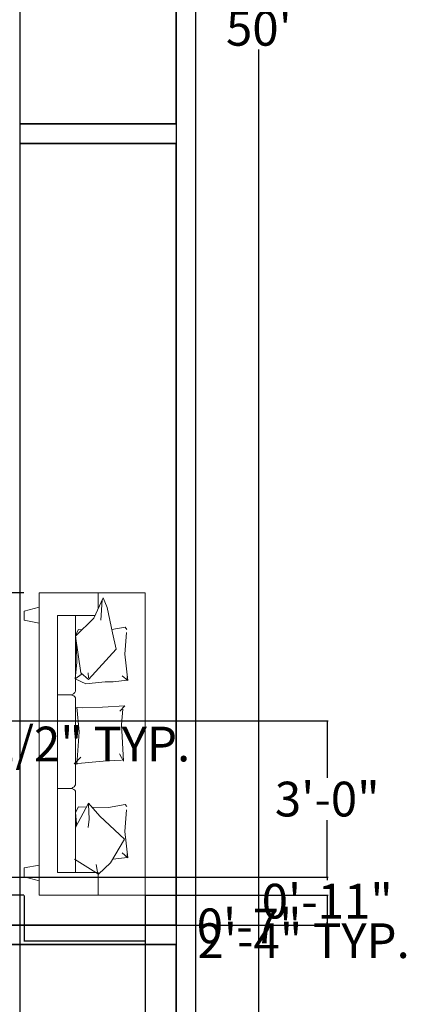
# Model space of a CAD drawing. Units: inches. Extents: x -26 to 385, y 12 to 697.
# Tile 11 of 13: x 285 to 374, y 130 to 356. Entities that reach past the tile are written whole.
import ezdxf

# ---------------------------------------------------------------- set-up
doc = ezdxf.new("R2010")
doc.units = ezdxf.units.IN
doc.header["$MEASUREMENT"] = 0
for name, color, linetype, lineweight in [('A-ANNO-DIMS', 4, 'Continuous', 18), ('A-FLOR-STRS', 215, 'Continuous', 18), ('A-WALL', 40, 'Continuous', 35), ('C-PROP', 40, 'Continuous', 25), ('Furniture', 210, 'Continuous', 15)]:
    doc.layers.add(name, color=color, linetype=linetype, lineweight=lineweight)
doc.styles.get("Standard").update_dxf_attribs({"font": 'italic8.shx'})
doc.dimstyles.get("Standard").update_dxf_attribs({"dimtxt": 8, "dimasz": 0.18, "dimexe": 0.18, "dimexo": 0.0625, "dimgap": 0.09, "dimtad": 0, "dimtih": 1, "dimtoh": 1, "dimdec": 4, "dimzin": 0, "dimdsep": 46, "dimlunit": 3, "dimtxsty": 'Standard', "dimcen": 0.09, "dimclrd": 2, "dimclre": 3, "dimclrt": 6, "dimadec": 0, "dimazin": 0, "dimtfac": 1, "dimtdec": 4, "dimtofl": 0, "dimtmove": 0, "dimatfit": 3, "dimfxl": 1, "dimtolj": 1, "dimtzin": 0, "dimarcsym": 0})

# ---------------------------------------------------------------- blocks, each defined once
blk = doc.blocks.new('*D2')
at = {"layer": 'A-ANNO-DIMS', "color": 0, "lineweight": -2, "transparency": 16777216}
for p, q in [((325.19, 654.38), (339.84, 654.38)), ((339.66, 654.2), (339.66, 359.23)), ((339.66, 54.56), (339.66, 349.53)), ((325.19, 54.38), (339.84, 54.38))]:
    blk.add_line(p, q, dxfattribs=at)
at = {"layer": 'A-ANNO-DIMS', "color": 0, "transparency": 16777216}
for points in [[(339.63, 654.2), (339.69, 654.2), (339.66, 654.38)], [(339.63, 54.56), (339.69, 54.56), (339.66, 54.38)]]:
    blk.add_solid(points, dxfattribs=at)
at = {"layer": 'Defpoints', "color": 0, "transparency": 16777216}
for p in [(325.13, 654.38), (325.13, 54.38), (339.66, 54.38)]:
    blk.add_point(p, dxfattribs=at)
at = {"layer": 'A-ANNO-DIMS', "color": 0, "transparency": 16777216, "insert": (339.66, 354.38), "char_height": 8, "attachment_point": 5}
blk.add_mtext("\\A1;50'", dxfattribs=at)
blk = doc.blocks.new('SOFA-THREE-SEAT')
for p, q in [((-5.22, 20.2), (64.44, 20.2)), ((-5.22, 20.2), (-5.22, -4.18)), ((64.44, 20.2), (64.44, -4.18)), ((2.7, 15.63), (3.2, 15.97)), ((3.92, 15.91), (8.89, 15.54)), ((8.89, 15.54), (14.99, 16.19)), ((14.99, 16.19), (13.87, 14.88)), ((14.06, 16.09), (14.9, 16.1)), ((14.9, 16.1), (15.27, 12.82)), ((43.52, 15.63), (44.02, 15.97)), ((44.74, 15.91), (49.71, 15.54)), ((49.71, 15.54), (55.81, 16.19)), ((55.81, 16.19), (54.69, 14.88)), ((54.88, 16.09), (55.72, 16.1)), ((55.72, 16.1), (56.09, 12.82)), ((3.23, 12.52), (2.7, 15.63)), ((21.11, 10.37), (20.83, 15.51)), ((20.83, 15.51), (22.04, 14.39)), ((21.58, 15.04), (25.13, 14.76)), ((25.13, 14.76), (33.53, 15.23)), ((33.53, 15.23), (31.85, 14.29)), ((33.35, 14.76), (33.44, 11.4)), ((44.18, 11.79), (43.52, 15.63)), ((46.2, 9.78), (51.51, 15.49)), ((51.51, 15.49), (56.95, 12.22)), ((-1.8, 11.46), (-4.04, 10.53)), ((3.97, 12.67), (-1.8, 11.46)), ((7.78, 13.51), (3.97, 12.67)), ((14.76, 7.19), (7.78, 13.51)), ((15.27, 12.82), (15.27, 11.04)), ((33.44, 11.4), (34.19, 3.84)), ((44.12, 7.99), (44.18, 11.79)), ((56.09, 12.82), (56.09, 12.74)), ((56.95, 12.22), (59.54, 9.5)), ((-5.22, 9.4), (-1.58, 9.4)), ((-4.04, 10.53), (0.62, 8.39)), ((-3.57, 10.35), (1.08, 9.97)), ((15.27, 11.04), (15.74, 6.54)), ((21.3, 5.71), (21.11, 10.37)), ((43.2, 7.19), (46.2, 9.78)), ((59.54, 9.5), (56.14, 3.93)), ((59.13, 9.23), (57.36, 8.96)), ((59.21, 9.4), (59.21, 0)), ((59.21, 9.4), (64.44, 9.4)), ((0, 8.68), (0, 0)), ((0.62, 8.39), (4.8, 4.21)), ((14.39, 7.19), (13.18, 7.09)), ((13.18, 5.42), (14.76, 7.19)), ((48.79, 4.2), (43.2, 7.19)), ((43.48, 7.19), (46.88, 7.33)), ((46.88, 7.33), (48.79, 7.06)), ((3.26, 4.85), (3.27, 5.74)), ((4.57, 4.19), (3.26, 4.85)), ((4.8, 4.21), (13.18, 5.42)), ((14.62, 4.1), (13.47, 5.75)), ((15.74, 6.54), (14.62, 4.1)), ((21.11, 4.5), (26.81, 5.06)), ((21.2, 4.4), (21.3, 5.71)), ((26.81, 5.06), (34.28, 4.5)), ((34.19, 3.84), (32.6, 5.43)), ((44.08, 4.85), (44.11, 6.71)), ((45.4, 4.19), (44.08, 4.85)), ((0, 4.18), (17.44, 4.18)), ((7.11, 4.38), (4.57, 4.19)), ((10.86, 4.47), (7.11, 4.38)), ((14.62, 4.1), (10.86, 4.47)), ((18.3, 3.23), (18.3, 0)), ((18.93, 4.18), (38.96, 4.18)), ((39.82, 3.23), (39.82, 0)), ((40.44, 4.18), (59.21, 4.18)), ((47.93, 4.38), (45.4, 4.19)), ((48.43, 4.39), (47.93, 4.38)), ((0, 0), (59.21, 0)), ((-5.22, -4.18), (64.44, -4.18)), ((-1.91, -4.18), (-1.01, -7.66)), ((1.75, -4.18), (1.07, -7.66)), ((57.47, -4.18), (58.14, -7.66)), ((61.12, -4.18), (60.22, -7.66)), ((-1.01, -7.66), (1.07, -7.66)), ((58.14, -7.66), (60.22, -7.66))]:
    blk.add_line(p, q)
for points, knots in [([(17.44, 4.18), (17.62, 4.1), (18, 3.87), (18.2, 3.46), (18.3, 3.23)], [15.247039, 15.247039, 15.247039, 15.247039, 32.166322, 53.547435, 53.547435, 53.547435, 53.547435]), ([(18.3, 3.22), (18.36, 3.42), (18.48, 3.8), (18.78, 4.06), (18.93, 4.18)], [5.353258, 5.353258, 5.353258, 5.353258, 23.098733, 39.167876, 39.167876, 39.167876, 39.167876]), ([(38.96, 4.18), (39.14, 4.1), (39.51, 3.87), (39.71, 3.46), (39.82, 3.23)], [15.247039, 15.247039, 15.247039, 15.247039, 32.166322, 53.547435, 53.547435, 53.547435, 53.547435]), ([(39.82, 3.22), (39.87, 3.42), (39.99, 3.8), (40.29, 4.06), (40.44, 4.18)], [5.353258, 5.353258, 5.353258, 5.353258, 23.098733, 39.167876, 39.167876, 39.167876, 39.167876])]:
    blk.add_open_spline(points, degree=3, knots=knots)
blk = doc.blocks.new('*D11')
at = {"layer": 'A-ANNO-DIMS', "color": 3, "lineweight": -2, "transparency": 16777216}
for p, q in [((285.56, 224.4), (274.99, 224.4)), ((285.56, 154.74), (274.99, 154.74))]:
    blk.add_line(p, q, dxfattribs=at)
at = {"layer": 'A-ANNO-DIMS', "color": 2, "lineweight": -2, "transparency": 16777216}
for p, q in [((275.17, 224.22), (275.17, 195.75)), ((275.17, 154.92), (275.17, 183.38))]:
    blk.add_line(p, q, dxfattribs=at)
at = {"layer": 'A-ANNO-DIMS', "color": 2, "transparency": 16777216}
for points in [[(275.14, 224.22), (275.2, 224.22), (275.17, 224.4)], [(275.14, 154.92), (275.2, 154.92), (275.17, 154.74)]]:
    blk.add_solid(points, dxfattribs=at)
at = {"layer": 'Defpoints', "color": 0, "transparency": 16777216}
for p in [(285.62, 224.4), (275.17, 154.74), (285.62, 154.74)]:
    blk.add_point(p, dxfattribs=at)
at = {"layer": 'A-ANNO-DIMS', "color": 6, "transparency": 16777216, "insert": (275.17, 189.57), "char_height": 8, "attachment_point": 5}
blk.add_mtext('\\A1;SOFA 5\'-9 1/2" TYP.', dxfattribs=at)
blk = doc.blocks.new('*D12')
at = {"layer": 'A-ANNO-DIMS', "color": 3, "lineweight": -2, "transparency": 16777216}
for p, q in [((285.62, 154.68), (285.62, 144.11)), ((313.49, 154.68), (313.49, 144.11))]:
    blk.add_line(p, q, dxfattribs=at)
at = {"layer": 'A-ANNO-DIMS', "color": 2, "lineweight": -2, "transparency": 16777216}
for p, q in [((285.8, 144.29), (313.31, 144.29)), ((313.49, 144.29), (313.67, 144.29))]:
    blk.add_line(p, q, dxfattribs=at)
at = {"layer": 'A-ANNO-DIMS', "color": 2, "transparency": 16777216}
for points in [[(285.8, 144.32), (285.8, 144.26), (285.62, 144.29)], [(313.31, 144.32), (313.31, 144.26), (313.49, 144.29)]]:
    blk.add_solid(points, dxfattribs=at)
at = {"layer": 'Defpoints', "color": 0, "transparency": 16777216}
for p in [(285.62, 154.74), (313.49, 154.74), (313.49, 144.29)]:
    blk.add_point(p, dxfattribs=at)
at = {"layer": 'A-ANNO-DIMS', "color": 6, "transparency": 16777216, "insert": (349.95, 144.29), "char_height": 8, "attachment_point": 5}
blk.add_mtext('\\A1;2\'-4" TYP.', dxfattribs=at)
blk = doc.blocks.new('*D25')
at = {"layer": 'A-ANNO-DIMS', "color": 3, "lineweight": -2, "transparency": 16777216}
for p, q in [((284.629322, 368.316588), (284.629322, 23.949088)), ((320.629322, 368.316588), (320.629322, 23.949088))]:
    blk.add_line(p, q, dxfattribs=at)
at = {"layer": 'A-ANNO-DIMS', "color": 2, "lineweight": -2, "transparency": 16777216}
for p, q in [((284.449322, 24.129088), (284.269322, 24.129088)), ((320.809322, 24.129088), (320.989322, 24.129088))]:
    blk.add_line(p, q, dxfattribs=at)
at = {"layer": 'A-ANNO-DIMS', "color": 2, "transparency": 16777216}
for points in [[(284.449322, 24.159088), (284.449322, 24.099088), (284.629322, 24.129088)], [(320.809322, 24.159088), (320.809322, 24.099088), (320.629322, 24.129088)]]:
    blk.add_solid(points, dxfattribs=at)
at = {"layer": 'Defpoints', "color": 0, "transparency": 16777216}
for p in [(284.629322, 368.379088), (320.629322, 368.379088), (320.629322, 24.129088)]:
    blk.add_point(p, dxfattribs=at)
at = {"layer": 'A-ANNO-DIMS', "color": 6, "transparency": 16777216, "insert": (302.629322, 24.129088), "char_height": 8, "attachment_point": 5}
blk.add_mtext('\\A1;3\'-0"', dxfattribs=at)
blk = doc.blocks.new('*D28')
at = {"layer": 'A-ANNO-DIMS', "color": 3, "lineweight": -2, "transparency": 16777216}
for p, q in [((141.69, 194.9), (355.56, 194.9)), ((141.69, 158.9), (355.56, 158.9))]:
    blk.add_line(p, q, dxfattribs=at)
at = {"layer": 'A-ANNO-DIMS', "color": 2, "lineweight": -2, "transparency": 16777216}
for p, q in [((355.38, 194.72), (355.38, 181.76)), ((355.38, 159.08), (355.38, 172.05))]:
    blk.add_line(p, q, dxfattribs=at)
at = {"layer": 'A-ANNO-DIMS', "color": 2, "transparency": 16777216}
for points in [[(355.35, 194.72), (355.41, 194.72), (355.38, 194.9)], [(355.35, 159.08), (355.41, 159.08), (355.38, 158.9)]]:
    blk.add_solid(points, dxfattribs=at)
at = {"layer": 'Defpoints', "color": 0, "transparency": 16777216}
for p in [(141.63, 194.9), (355.38, 194.9), (141.63, 158.9)]:
    blk.add_point(p, dxfattribs=at)
at = {"layer": 'A-ANNO-DIMS', "color": 6, "transparency": 16777216, "insert": (355.38, 176.9), "char_height": 8, "attachment_point": 5}
blk.add_mtext('\\A1;3\'-0"', dxfattribs=at)
blk = doc.blocks.new('*D31')
at = {"layer": 'A-ANNO-DIMS', "color": 3, "lineweight": -2, "transparency": 16777216}
for p, q in [((239.89, 166.08), (239.89, 23.95)), ((263.51, 166.08), (263.51, 23.95))]:
    blk.add_line(p, q, dxfattribs=at)
at = {"layer": 'A-ANNO-DIMS', "color": 2, "lineweight": -2, "transparency": 16777216}
for p, q in [((240.07, 24.13), (263.33, 24.13)), ((263.51, 24.13), (263.69, 24.13))]:
    blk.add_line(p, q, dxfattribs=at)
at = {"layer": 'A-ANNO-DIMS', "color": 2, "transparency": 16777216}
for points in [[(240.07, 24.16), (240.07, 24.1), (239.89, 24.13)], [(263.33, 24.16), (263.33, 24.1), (263.51, 24.13)]]:
    blk.add_solid(points, dxfattribs=at)
at = {"layer": 'Defpoints', "color": 0, "transparency": 16777216}
for p in [(239.89, 166.14), (263.51, 166.14), (263.51, 24.13)]:
    blk.add_point(p, dxfattribs=at)
at = {"layer": 'A-ANNO-DIMS', "color": 6, "transparency": 16777216, "insert": (296.73, 24.13), "char_height": 8, "attachment_point": 5}
blk.add_mtext('\\A1;1\'-11 1/2"', dxfattribs=at)
blk = doc.blocks.new('*D35')
at = {"layer": 'A-ANNO-DIMS', "color": 3, "lineweight": -2, "transparency": 16777216}
for p, q in [((193.6, 147.94), (193.6, 684.81)), ((244.99, 147.94), (244.99, 684.81))]:
    blk.add_line(p, q, dxfattribs=at)
at = {"layer": 'A-ANNO-DIMS', "color": 2, "lineweight": -2, "transparency": 16777216}
for p, q in [((193.78, 684.63), (244.81, 684.63)), ((244.99, 684.63), (245.17, 684.63))]:
    blk.add_line(p, q, dxfattribs=at)
at = {"layer": 'A-ANNO-DIMS', "color": 2, "transparency": 16777216}
for points in [[(193.78, 684.66), (193.78, 684.6), (193.6, 684.63)], [(244.81, 684.66), (244.81, 684.6), (244.99, 684.63)]]:
    blk.add_solid(points, dxfattribs=at)
at = {"layer": 'Defpoints', "color": 0, "transparency": 16777216}
for p in [(244.99, 684.63), (193.6, 147.88), (244.99, 147.88)]:
    blk.add_point(p, dxfattribs=at)
at = {"layer": 'A-ANNO-DIMS', "color": 6, "transparency": 16777216, "insert": (278.4, 684.63), "char_height": 8, "attachment_point": 5}
blk.add_mtext('\\A1;4\'-3 1/2"', dxfattribs=at)
blk = doc.blocks.new('*D37')
at = {"layer": 'A-ANNO-DIMS', "color": 3, "lineweight": -2, "transparency": 16777216}
for p, q in [((223.55, 597.32), (223.55, 23.95)), ((257.22, 597.32), (257.22, 23.95))]:
    blk.add_line(p, q, dxfattribs=at)
at = {"layer": 'A-ANNO-DIMS', "color": 2, "lineweight": -2, "transparency": 16777216}
for p, q in [((223.73, 24.13), (257.04, 24.13)), ((257.22, 24.13), (257.4, 24.13))]:
    blk.add_line(p, q, dxfattribs=at)
at = {"layer": 'A-ANNO-DIMS', "color": 2, "transparency": 16777216}
for points in [[(223.73, 24.16), (223.73, 24.1), (223.55, 24.13)], [(257.04, 24.16), (257.04, 24.1), (257.22, 24.13)]]:
    blk.add_solid(points, dxfattribs=at)
at = {"layer": 'Defpoints', "color": 0, "transparency": 16777216}
for p in [(223.55, 597.38), (257.22, 597.38), (257.22, 24.13)]:
    blk.add_point(p, dxfattribs=at)
at = {"layer": 'A-ANNO-DIMS', "color": 6, "transparency": 16777216, "insert": (290.63, 24.13), "char_height": 8, "attachment_point": 5}
blk.add_mtext('\\A1;2\'-9 1/2"', dxfattribs=at)
blk = doc.blocks.new('*D42')
at = {"layer": 'A-ANNO-DIMS', "color": 3, "lineweight": -2, "transparency": 16777216}
for p, q in [((250.37, 518.99), (250.37, 23.95)), ((274.13, 518.99), (274.13, 23.95))]:
    blk.add_line(p, q, dxfattribs=at)
at = {"layer": 'A-ANNO-DIMS', "color": 2, "lineweight": -2, "transparency": 16777216}
for p, q in [((250.55, 24.13), (273.95, 24.13)), ((274.13, 24.13), (274.31, 24.13))]:
    blk.add_line(p, q, dxfattribs=at)
at = {"layer": 'A-ANNO-DIMS', "color": 2, "transparency": 16777216}
for points in [[(250.55, 24.16), (250.55, 24.1), (250.37, 24.13)], [(273.95, 24.16), (273.95, 24.1), (274.13, 24.13)]]:
    blk.add_solid(points, dxfattribs=at)
at = {"layer": 'Defpoints', "color": 0, "transparency": 16777216}
for p in [(250.37, 519.05), (274.13, 519.05), (274.13, 24.13)]:
    blk.add_point(p, dxfattribs=at)
at = {"layer": 'A-ANNO-DIMS', "color": 6, "transparency": 16777216, "insert": (292.3, 24.13), "char_height": 8, "attachment_point": 5}
blk.add_mtext('\\A1;2\'-0"', dxfattribs=at)
blk = doc.blocks.new('*D50')
at = {"layer": 'A-ANNO-DIMS', "color": 3, "lineweight": -2, "transparency": 16777216}
for p, q in [((246.28, 401.87), (246.28, 23.95)), ((284.63, 398.32), (284.63, 23.95))]:
    blk.add_line(p, q, dxfattribs=at)
at = {"layer": 'A-ANNO-DIMS', "color": 2, "lineweight": -2, "transparency": 16777216}
for p, q in [((246.46, 24.13), (284.45, 24.13)), ((284.63, 24.13), (284.81, 24.13))]:
    blk.add_line(p, q, dxfattribs=at)
at = {"layer": 'A-ANNO-DIMS', "color": 2, "transparency": 16777216}
for points in [[(246.46, 24.16), (246.46, 24.1), (246.28, 24.13)], [(284.45, 24.16), (284.45, 24.1), (284.63, 24.13)]]:
    blk.add_solid(points, dxfattribs=at)
at = {"layer": 'Defpoints', "color": 0, "transparency": 16777216}
for p in [(246.28, 401.93), (284.63, 398.38), (284.63, 24.13)]:
    blk.add_point(p, dxfattribs=at)
at = {"layer": 'A-ANNO-DIMS', "color": 6, "transparency": 16777216, "insert": (318.04, 24.13), "char_height": 8, "attachment_point": 5}
blk.add_mtext('\\A1;3\'-2 1/2"', dxfattribs=at)
blk = doc.blocks.new('*D52')
at = {"layer": 'A-ANNO-DIMS', "color": 3, "lineweight": -2, "transparency": 16777216}
for p, q in [((313.49, 154.68), (313.49, 23.95)), ((320.63, 147.82), (320.63, 23.95))]:
    blk.add_line(p, q, dxfattribs=at)
at = {"layer": 'A-ANNO-DIMS', "color": 2, "lineweight": -2, "transparency": 16777216}
for p, q in [((313.67, 24.13), (320.45, 24.13)), ((320.63, 24.13), (320.81, 24.13))]:
    blk.add_line(p, q, dxfattribs=at)
at = {"layer": 'A-ANNO-DIMS', "color": 2, "transparency": 16777216}
for points in [[(313.67, 24.16), (313.67, 24.1), (313.49, 24.13)], [(320.45, 24.16), (320.45, 24.1), (320.63, 24.13)]]:
    blk.add_solid(points, dxfattribs=at)
at = {"layer": 'Defpoints', "color": 0, "transparency": 16777216}
for p in [(313.49, 154.74), (320.63, 147.88), (320.63, 24.13)]:
    blk.add_point(p, dxfattribs=at)
at = {"layer": 'A-ANNO-DIMS', "color": 6, "transparency": 16777216, "insert": (338.61, 24.13), "char_height": 8, "attachment_point": 5}
blk.add_mtext('\\A1;0\'-7"', dxfattribs=at)
blk = doc.blocks.new('*D53')
at = {"layer": 'A-ANNO-DIMS', "color": 3, "lineweight": -2, "transparency": 16777216}
for p, q in [((313.55, 154.74), (355.56, 154.74)), ((320.69, 147.88), (355.56, 147.88))]:
    blk.add_line(p, q, dxfattribs=at)
at = {"layer": 'A-ANNO-DIMS', "color": 2, "lineweight": -2, "transparency": 16777216}
for p, q in [((355.38, 154.56), (355.38, 148.06)), ((355.38, 147.7), (355.2, 147.7)), ((355.38, 147.88), (355.38, 147.7))]:
    blk.add_line(p, q, dxfattribs=at)
at = {"layer": 'A-ANNO-DIMS', "color": 2, "transparency": 16777216}
for points in [[(355.35, 154.56), (355.41, 154.56), (355.38, 154.74)], [(355.35, 148.06), (355.41, 148.06), (355.38, 147.88)]]:
    blk.add_solid(points, dxfattribs=at)
at = {"layer": 'Defpoints', "color": 0, "transparency": 16777216}
for p in [(313.49, 154.74), (320.63, 147.88), (355.38, 147.88)]:
    blk.add_point(p, dxfattribs=at)
at = {"layer": 'A-ANNO-DIMS', "color": 6, "transparency": 16777216, "insert": (337.4, 147.7), "char_height": 8, "attachment_point": 5}
blk.add_mtext('\\A1;0\'-7"', dxfattribs=at)
blk = doc.blocks.new('*D55')
at = {"layer": 'A-ANNO-DIMS', "color": 3, "lineweight": -2, "transparency": 16777216}
for p, q in [((146.19, 158.9), (355.56, 158.9)), ((146.19, 147.88), (355.56, 147.88))]:
    blk.add_line(p, q, dxfattribs=at)
at = {"layer": 'A-ANNO-DIMS', "color": 2, "lineweight": -2, "transparency": 16777216}
for p, q in [((355.38, 158.72), (355.38, 158.24)), ((355.38, 148.06), (355.38, 148.54))]:
    blk.add_line(p, q, dxfattribs=at)
at = {"layer": 'A-ANNO-DIMS', "color": 2, "transparency": 16777216}
for points in [[(355.35, 158.72), (355.41, 158.72), (355.38, 158.9)], [(355.35, 148.06), (355.41, 148.06), (355.38, 147.88)]]:
    blk.add_solid(points, dxfattribs=at)
at = {"layer": 'Defpoints', "color": 0, "transparency": 16777216}
for p in [(146.13, 158.9), (355.38, 158.9), (146.13, 147.88)]:
    blk.add_point(p, dxfattribs=at)
at = {"layer": 'A-ANNO-DIMS', "color": 6, "transparency": 16777216, "insert": (355.38, 153.39), "char_height": 8, "attachment_point": 5}
blk.add_mtext('\\A1;0\'-11"', dxfattribs=at)

msp = doc.modelspace()

# ---------------------------------------------------------------- linework, layer by layer
at = {"layer": 'A-FLOR-STRS'}
msp.add_line((284.62932, 327.87909), (284.62932, 477.37909), dxfattribs=at)
at = {"layer": 'A-WALL'}
for p, q in [((320.62932, 332.37909), (320.62932, 477.37909)), ((320.62932, 332.37909), (284.62932, 332.37909)), ((320.62932, 327.87909), (284.62932, 327.87909)), ((320.62932, 147.87909), (320.62932, 327.87909)), ((320.62932, 147.87909), (146.12932, 147.87909)), ((320.62932, 143.37909), (141.62932, 143.37909)), ((320.62932, 58.87909), (320.62932, 143.37909))]:
    msp.add_line(p, q, dxfattribs=at)
at = {"layer": 'C-PROP'}
msp.add_line((325.12932, 54.37909), (325.12932, 654.37909), dxfattribs=at)

# ---------------------------------------------------------------- block references
at = {"layer": 'Furniture', "rotation": 269.9999999999995}
msp.add_blockref('SOFA-THREE-SEAT', (293.28536, 219.17697), dxfattribs=at)

# ---------------------------------------------------------------- dimensions: what is measured, and where the dimension line sits
at = {"layer": 'A-ANNO-DIMS'}
for base, p1, p2, picture, middle in [((244.98557, 684.62909), (193.59818, 147.87909), (244.98557, 147.87909), '*D35', (278.39843, 684.62909)), ((257.21981, 24.12909), (223.54856, 597.37909), (257.21981, 597.37909), '*D37', (290.63267, 24.12909)), ((274.12932, 24.12909), (250.37102, 519.05498), (274.12932, 519.05498), '*D42', (292.30408, 24.12909)), ((284.62932, 24.12909), (246.27828, 401.934), (284.62932, 398.37909), '*D50', (318.04218, 24.12909)), ((320.62932, 24.12909), (284.62932, 368.37909), (320.62932, 368.37909), '*D25', (302.62932, 24.12909)), ((263.50956, 24.12909), (239.88756, 166.14113), (263.50956, 166.14113), '*D31', (296.73194, 24.12909)), ((320.62932, 24.12909), (313.48771, 154.73754), (320.62932, 147.87909), '*D52', (338.61361, 24.12909))]:
    dim = msp.add_linear_dim(base=base, p1=p1, p2=p2, dimstyle='Standard', override={"dimdec": 1, "dimlfac": 1, "dimrnd": 0, "dimzin": 1, "dimdsep": 46, "dimlunit": 4, "dimfrac": 2}, dxfattribs=at)
    dim.commit()
    dim.dimension.update_dxf_attribs({"geometry": picture, "text_midpoint": middle})
for base, p1, p2, override, picture, middle in [((339.65968, 54.37909), (325.12932, 654.37909), (325.12932, 54.37909), {"dimclrd": 0, "dimclre": 0, "dimclrt": 0}, '*D2', (339.65968, 354.37909)), ((355.37932, 194.90341), (141.62932, 158.90341), (141.62932, 194.90341), {"dimdec": 1, "dimlfac": 1, "dimrnd": 0, "dimzin": 1, "dimdsep": 46, "dimlunit": 4, "dimfrac": 2}, '*D28', (355.37932, 176.90341)), ((355.37932, 158.90341), (146.12932, 147.87909), (146.12932, 158.90341), {"dimdec": 1, "dimlfac": 1, "dimrnd": 0, "dimzin": 1, "dimdsep": 46, "dimlunit": 4, "dimfrac": 2}, '*D55', (355.37932, 153.39125)), ((355.37932, 147.87909), (313.48771, 154.73754), (320.62932, 147.87909), {"dimdec": 1, "dimlfac": 1, "dimrnd": 0, "dimzin": 1, "dimdsep": 46, "dimlunit": 4, "dimfrac": 2}, '*D53', (337.39504, 147.69909))]:
    dim = msp.add_linear_dim(base=base, p1=p1, p2=p2, angle=90, dimstyle='Standard', override=override, dxfattribs=at)
    dim.commit()
    dim.dimension.update_dxf_attribs({"geometry": picture, "text_midpoint": middle})
dim = msp.add_linear_dim(base=(275.17245, 154.73754), p1=(285.62207, 224.40165), p2=(285.62207, 154.73754), angle=270, text='SOFA <> TYP.', dimstyle='Standard', override={"dimdec": 1, "dimlfac": 1, "dimrnd": 0, "dimzin": 1, "dimdsep": 46, "dimlunit": 4, "dimfrac": 2}, dxfattribs=at)
dim.commit()
dim.dimension.update_dxf_attribs({"geometry": '*D11', "text_midpoint": (275.17245, 189.56959)})
dim = msp.add_linear_dim(base=(313.48771, 144.28792), p1=(285.62207, 154.73754), p2=(313.48771, 154.73754), text='<> TYP.', dimstyle='Standard', override={"dimdec": 1, "dimlfac": 1, "dimrnd": 0, "dimzin": 1, "dimdsep": 46, "dimlunit": 4, "dimfrac": 2}, dxfattribs=at)
dim.commit()
dim.dimension.update_dxf_attribs({"geometry": '*D12', "text_midpoint": (349.94819, 144.28792)})

doc.saveas('drawing.dxf')
